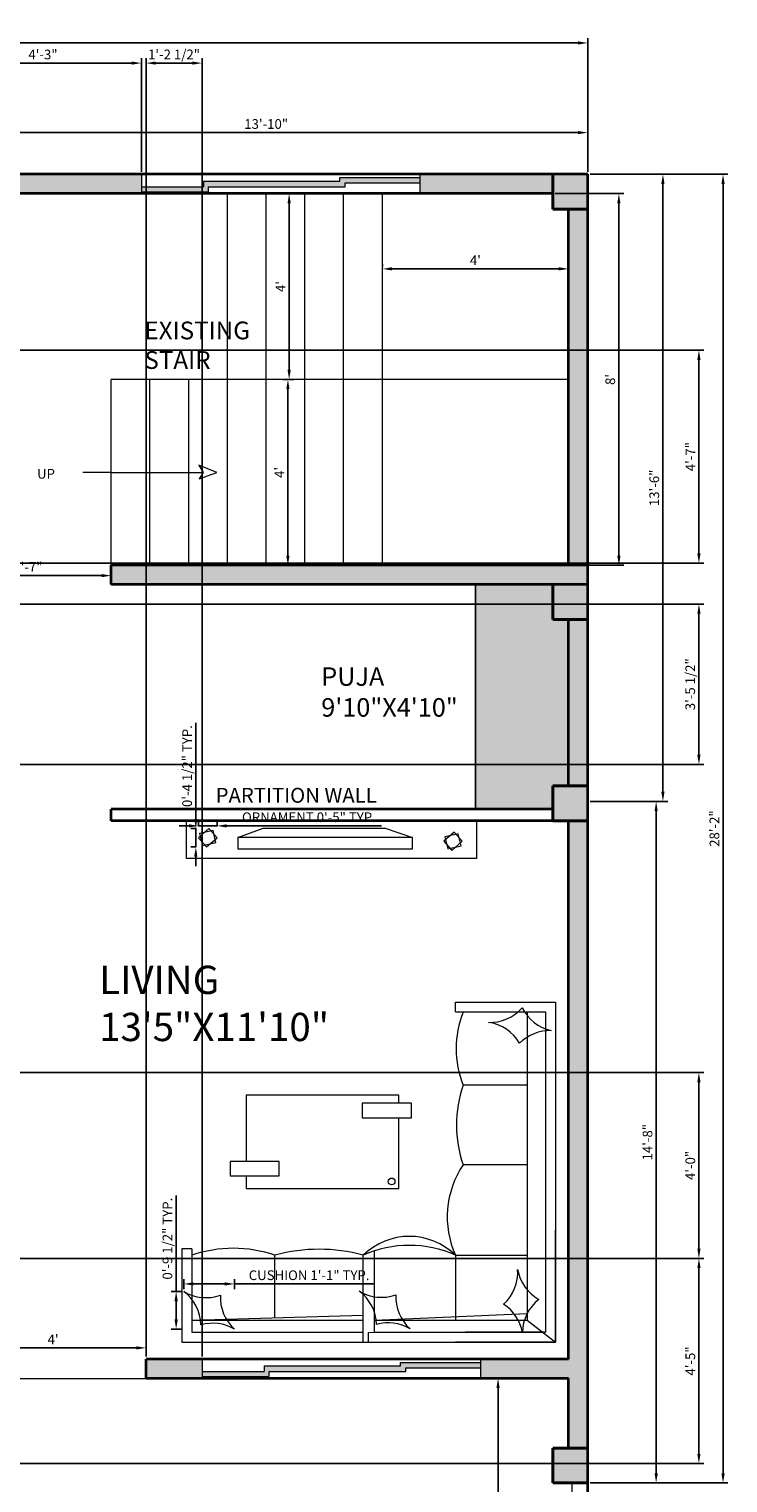
# Model space of a CAD drawing. Units: inches. Extents: x 918 to 1328, y 603 to 1174.
# Tile 4 of 4: x 1147 to 1328, y 798 to 1174. Entities that reach past the tile are written whole.
import ezdxf

# ---------------------------------------------------------------- set-up
doc = ezdxf.new("R2010")
doc.units = ezdxf.units.IN
for name, color, linetype, lineweight in [('A-ANNO-DIMS', 1, 'Continuous', 18), ('A-ANNO-SYMB', 1, 'Continuous', 18), ('A-ANNO-TEXT', 7, 'Continuous', 18), ('A-COLS', 7, 'Continuous', 40), ('A-DOOR', 4, 'Continuous', 18), ('A-FLOR', 7, 'Continuous', 25), ('A-FLOR-CASE', 8, 'Continuous', 20), ('A-FLOR-RAIL', 7, 'Continuous', 18), ('A-FURN', 8, 'Continuous', 18), ('A-GLAZ', 4, 'Continuous', 18), ('A-GLAZ-PATT', 5, 'Continuous', 13), ('A-WALL', 7, 'Continuous', 35), ('A-WALL-PATT', 7, 'Continuous', 13)]:
    doc.layers.add(name, color=color, linetype=linetype, lineweight=lineweight)
for name, color, linetype, lineweight, true_color in [('A-AREA-IDEN', 251, 'Continuous', 20, 0x636466), ('A-COLS-PATT', 251, 'Continuous', 13, 0x636466), ('A-EQPM', 252, 'Continuous', 18, 0x939598), ('A-FLOR-PATT', 40, 'Continuous', 13, 0xf8d731), ('A-FLOR-STRS', 251, 'Continuous', 20, 0x636466)]:
    doc.layers.add(name, color=color, linetype=linetype, lineweight=lineweight, true_color=true_color)
doc.styles.get("Standard").update_dxf_attribs({"font": 'arial.ttf'})
doc.dimstyles.new('ISO-25', dxfattribs={"dimtxt": 2.5, "dimasz": 2.5, "dimexe": 1.25, "dimexo": 0.625, "dimtad": 1, "dimdec": 0, "dimlunit": 3, "dimtxsty": 'Standard', "dimcen": 2.5, "dimadec": 0, "dimazin": 0, "dimtfac": 1, "dimtdec": 0, "dimtmove": 0, "dimatfit": 3, "dimfxl": 1, "dimarcsym": 0})

# ---------------------------------------------------------------- blocks, each defined once
blk = doc.blocks.new('*D1')
at = {"layer": 'A-ANNO-DIMS', "color": 0, "lineweight": -2, "transparency": 16777216}
for p, q in [((956.48, 1136.87), (956.48, 1171.39)), ((958.98, 1170.14), (1288.98, 1170.14)), ((1291.48, 1136.87), (1291.48, 1171.39))]:
    blk.add_line(p, q, dxfattribs=at)
at = {"layer": 'A-ANNO-DIMS', "color": 0, "transparency": 16777216}
for points in [[(958.98, 1170.56), (958.98, 1169.73), (956.48, 1170.14)], [(1288.98, 1170.56), (1288.98, 1169.73), (1291.48, 1170.14)]]:
    blk.add_solid(points, dxfattribs=at)
at = {"layer": 'Defpoints', "color": 0, "transparency": 16777216}
for p in [(1291.48, 1170.14), (956.48, 1136.24), (1291.48, 1136.24)]:
    blk.add_point(p, dxfattribs=at)
at = {"layer": 'A-ANNO-DIMS', "color": 0, "transparency": 16777216, "insert": (1123.98, 1172.02), "char_height": 2.5, "attachment_point": 5}
blk.add_mtext('27\'-11"', dxfattribs=at)
blk = doc.blocks.new('*D4')
at = {"layer": 'A-ANNO-DIMS', "color": 0, "lineweight": -2, "transparency": 16777216}
for p, q in [((1292.11, 1136.24), (1327.66, 1136.24)), ((1326.41, 800.74), (1326.41, 1133.74)), ((1292.11, 798.24), (1327.66, 798.24))]:
    blk.add_line(p, q, dxfattribs=at)
at = {"layer": 'A-ANNO-DIMS', "color": 0, "transparency": 16777216}
for points in [[(1326, 1133.74), (1326.83, 1133.74), (1326.41, 1136.24)], [(1326, 800.74), (1326.83, 800.74), (1326.41, 798.24)]]:
    blk.add_solid(points, dxfattribs=at)
at = {"layer": 'Defpoints', "color": 0, "transparency": 16777216}
for p in [(1291.48, 1136.24), (1326.41, 1136.24), (1291.48, 798.24)]:
    blk.add_point(p, dxfattribs=at)
at = {"layer": 'A-ANNO-DIMS', "color": 0, "transparency": 16777216, "insert": (1324.51, 967.24), "char_height": 2.5, "attachment_point": 5, "rotation": 90}
blk.add_mtext('28\'-2"', dxfattribs=at)
blk = doc.blocks.new('*D5')
at = {"layer": 'A-ANNO-DIMS', "color": 0, "lineweight": -2, "transparency": 16777216}
for p, q in [((1125.48, 1136.87), (1125.48, 1148.24)), ((1127.98, 1146.99), (1288.98, 1146.99)), ((1291.48, 1136.87), (1291.48, 1148.24))]:
    blk.add_line(p, q, dxfattribs=at)
at = {"layer": 'A-ANNO-DIMS', "color": 0, "transparency": 16777216}
for points in [[(1127.98, 1147.4), (1127.98, 1146.57), (1125.48, 1146.99)], [(1288.98, 1147.4), (1288.98, 1146.57), (1291.48, 1146.99)]]:
    blk.add_solid(points, dxfattribs=at)
at = {"layer": 'Defpoints', "color": 0, "transparency": 16777216}
for p in [(1291.48, 1146.99), (1125.48, 1136.24), (1291.48, 1136.24)]:
    blk.add_point(p, dxfattribs=at)
at = {"layer": 'A-ANNO-DIMS', "color": 0, "transparency": 16777216, "insert": (1208.48, 1148.89), "char_height": 2.5, "attachment_point": 5}
blk.add_mtext('13\'-10"', dxfattribs=at)
blk = doc.blocks.new('*D9')
at = {"layer": 'A-ANNO-DIMS', "color": 0, "lineweight": -2, "transparency": 16777216}
for p, q in [((1292.11, 1136.24), (1312.14, 1136.24)), ((1310.89, 976.74), (1310.89, 1133.74)), ((1292.11, 974.24), (1312.14, 974.24))]:
    blk.add_line(p, q, dxfattribs=at)
at = {"layer": 'A-ANNO-DIMS', "color": 0, "transparency": 16777216}
for points in [[(1310.47, 1133.74), (1311.3, 1133.74), (1310.89, 1136.24)], [(1310.47, 976.74), (1311.3, 976.74), (1310.89, 974.24)]]:
    blk.add_solid(points, dxfattribs=at)
at = {"layer": 'Defpoints', "color": 0, "transparency": 16777216}
for p in [(1291.48, 1136.24), (1310.89, 1136.24), (1291.48, 974.24)]:
    blk.add_point(p, dxfattribs=at)
at = {"layer": 'A-ANNO-DIMS', "color": 0, "transparency": 16777216, "insert": (1308.98, 1055.24), "char_height": 2.5, "attachment_point": 5, "rotation": 90}
blk.add_mtext('13\'-6"', dxfattribs=at)
blk = doc.blocks.new('*D10')
at = {"layer": 'A-ANNO-DIMS', "color": 0, "lineweight": -2, "transparency": 16777216}
for p, q in [((1292.11, 974.24), (1310.39, 974.24)), ((1309.14, 971.74), (1309.14, 800.74)), ((1292.11, 798.24), (1310.39, 798.24))]:
    blk.add_line(p, q, dxfattribs=at)
at = {"layer": 'A-ANNO-DIMS', "color": 0, "transparency": 16777216}
for points in [[(1308.73, 971.74), (1309.56, 971.74), (1309.14, 974.24)], [(1308.73, 800.74), (1309.56, 800.74), (1309.14, 798.24)]]:
    blk.add_solid(points, dxfattribs=at)
at = {"layer": 'Defpoints', "color": 0, "transparency": 16777216}
for p in [(1291.48, 974.24), (1291.48, 798.24), (1309.14, 798.24)]:
    blk.add_point(p, dxfattribs=at)
at = {"layer": 'A-ANNO-DIMS', "color": 0, "transparency": 16777216, "insert": (1307.24, 886.24), "char_height": 2.5, "attachment_point": 5, "rotation": 90}
blk.add_mtext('14\'-8"', dxfattribs=at)
blk = doc.blocks.new('*D12')
at = {"layer": 'A-ANNO-DIMS', "color": 0, "lineweight": -2, "transparency": 16777216}
for p, q in [((1283.11, 1131.24), (1300.77, 1131.24)), ((1299.52, 1128.74), (1299.52, 1037.74)), ((1283.11, 1035.24), (1300.77, 1035.24))]:
    blk.add_line(p, q, dxfattribs=at)
at = {"layer": 'A-ANNO-DIMS', "color": 0, "transparency": 16777216}
for points in [[(1299.11, 1128.74), (1299.94, 1128.74), (1299.52, 1131.24)], [(1299.11, 1037.74), (1299.94, 1037.74), (1299.52, 1035.24)]]:
    blk.add_solid(points, dxfattribs=at)
at = {"layer": 'Defpoints', "color": 0, "transparency": 16777216}
for p in [(1282.48, 1131.24), (1282.48, 1035.24), (1299.52, 1035.24)]:
    blk.add_point(p, dxfattribs=at)
at = {"layer": 'A-ANNO-DIMS', "color": 0, "transparency": 16777216, "insert": (1297.62, 1083.24), "char_height": 2.5, "attachment_point": 5, "rotation": 90}
blk.add_mtext("8'", dxfattribs=at)
blk = doc.blocks.new('*D13')
at = {"layer": 'A-ANNO-DIMS', "color": 0, "lineweight": -2, "transparency": 16777216}
for p, q in [((1238.48, 1112.43), (1238.48, 1113.05)), ((1240.98, 1111.8), (1283.98, 1111.8)), ((1286.48, 1112.43), (1286.48, 1113.05))]:
    blk.add_line(p, q, dxfattribs=at)
at = {"layer": 'A-ANNO-DIMS', "color": 0, "transparency": 16777216}
for points in [[(1240.98, 1112.22), (1240.98, 1111.38), (1238.48, 1111.8)], [(1283.98, 1112.22), (1283.98, 1111.38), (1286.48, 1111.8)]]:
    blk.add_solid(points, dxfattribs=at)
at = {"layer": 'Defpoints', "color": 0, "transparency": 16777216}
for p in [(1238.48, 1111.8), (1286.48, 1111.8), (1286.48, 1111.8)]:
    blk.add_point(p, dxfattribs=at)
at = {"layer": 'A-ANNO-DIMS', "color": 0, "transparency": 16777216, "insert": (1262.48, 1113.68), "char_height": 2.5, "attachment_point": 5}
blk.add_mtext("4'", dxfattribs=at)
blk = doc.blocks.new('*D14')
at = {"layer": 'A-ANNO-DIMS', "color": 0, "lineweight": -2, "transparency": 16777216}
for p, q in [((1214.22, 1131.24), (1215.66, 1131.24)), ((1214.41, 1085.74), (1214.41, 1128.74)), ((1214.22, 1083.24), (1215.66, 1083.24))]:
    blk.add_line(p, q, dxfattribs=at)
at = {"layer": 'A-ANNO-DIMS', "color": 0, "transparency": 16777216}
for points in [[(1213.99, 1128.74), (1214.83, 1128.74), (1214.41, 1131.24)], [(1213.99, 1085.74), (1214.83, 1085.74), (1214.41, 1083.24)]]:
    blk.add_solid(points, dxfattribs=at)
at = {"layer": 'Defpoints', "color": 0, "transparency": 16777216}
for p in [(1213.6, 1131.24), (1214.41, 1131.24), (1213.6, 1083.24)]:
    blk.add_point(p, dxfattribs=at)
at = {"layer": 'A-ANNO-DIMS', "color": 0, "transparency": 16777216, "insert": (1212.54, 1107.24), "char_height": 2.5, "attachment_point": 5, "rotation": 90}
blk.add_mtext("4'", dxfattribs=at)
blk = doc.blocks.new('*D15')
at = {"layer": 'A-ANNO-DIMS', "color": 0, "lineweight": -2, "transparency": 16777216}
for p, q in [((1213.79, 1083.24), (1212.84, 1083.24)), ((1214.09, 1080.74), (1214.09, 1037.74)), ((1213.79, 1035.24), (1212.84, 1035.24))]:
    blk.add_line(p, q, dxfattribs=at)
at = {"layer": 'A-ANNO-DIMS', "color": 0, "transparency": 16777216}
for points in [[(1213.67, 1080.74), (1214.5, 1080.74), (1214.09, 1083.24)], [(1213.67, 1037.74), (1214.5, 1037.74), (1214.09, 1035.24)]]:
    blk.add_solid(points, dxfattribs=at)
at = {"layer": 'Defpoints', "color": 0, "transparency": 16777216}
for p in [(1214.41, 1083.24), (1214.09, 1035.24), (1214.41, 1035.24)]:
    blk.add_point(p, dxfattribs=at)
at = {"layer": 'A-ANNO-DIMS', "color": 0, "transparency": 16777216, "insert": (1212.21, 1059.24), "char_height": 2.5, "attachment_point": 5, "rotation": 90}
blk.add_mtext("4'", dxfattribs=at)
blk = doc.blocks.new('*D16')
at = {"layer": 'A-ANNO-DIMS', "color": 0, "lineweight": -2, "transparency": 16777216}
for p, q in [((1125.48, 1033.2), (1125.48, 1033.82)), ((1168.48, 1033.2), (1168.48, 1033.82)), ((1165.98, 1032.57), (1127.98, 1032.57))]:
    blk.add_line(p, q, dxfattribs=at)
at = {"layer": 'A-ANNO-DIMS', "color": 0, "transparency": 16777216}
for points in [[(1127.98, 1032.99), (1127.98, 1032.16), (1125.48, 1032.57)], [(1165.98, 1032.99), (1165.98, 1032.16), (1168.48, 1032.57)]]:
    blk.add_solid(points, dxfattribs=at)
at = {"layer": 'Defpoints', "color": 0, "transparency": 16777216}
for p in [(1125.48, 1032.57), (1125.48, 1032.57), (1168.48, 1032.57)]:
    blk.add_point(p, dxfattribs=at)
at = {"layer": 'A-ANNO-DIMS', "color": 0, "transparency": 16777216, "insert": (1146.98, 1034.48), "char_height": 2.5, "attachment_point": 5}
blk.add_mtext('3\'-7"', dxfattribs=at)
blk = doc.blocks.new('*D17')
at = {"layer": 'A-ANNO-DIMS', "color": 0, "lineweight": -2, "transparency": 16777216}
for p, q in [((1129.48, 830.87), (1129.48, 834.37)), ((1177.48, 830.87), (1177.48, 834.37)), ((1131.98, 833.12), (1174.98, 833.12))]:
    blk.add_line(p, q, dxfattribs=at)
at = {"layer": 'A-ANNO-DIMS', "color": 0, "transparency": 16777216}
for points in [[(1131.98, 833.53), (1131.98, 832.7), (1129.48, 833.12)], [(1174.98, 833.53), (1174.98, 832.7), (1177.48, 833.12)]]:
    blk.add_solid(points, dxfattribs=at)
at = {"layer": 'Defpoints', "color": 0, "transparency": 16777216}
for p in [(1129.48, 830.24), (1177.48, 833.12), (1177.48, 830.24)]:
    blk.add_point(p, dxfattribs=at)
at = {"layer": 'A-ANNO-DIMS', "color": 0, "transparency": 16777216, "insert": (1153.48, 834.99), "char_height": 2.5, "attachment_point": 5}
blk.add_mtext("4'", dxfattribs=at)
blk = doc.blocks.new('*D20')
at = {"layer": 'A-ANNO-DIMS', "color": 0, "lineweight": -2, "transparency": 16777216}
for p, q in [((1272.05, 825.24), (1267.09, 825.24)), ((1268.34, 731.74), (1268.34, 822.74)), ((1272.05, 729.24), (1267.09, 729.24))]:
    blk.add_line(p, q, dxfattribs=at)
at = {"layer": 'A-ANNO-DIMS', "color": 0, "transparency": 16777216}
for points in [[(1267.92, 822.74), (1268.75, 822.74), (1268.34, 825.24)], [(1267.92, 731.74), (1268.75, 731.74), (1268.34, 729.24)]]:
    blk.add_solid(points, dxfattribs=at)
at = {"layer": 'Defpoints', "color": 0, "transparency": 16777216}
for p in [(1268.34, 825.24), (1272.68, 825.24), (1272.68, 729.24)]:
    blk.add_point(p, dxfattribs=at)
at = {"layer": 'A-ANNO-DIMS', "color": 0, "transparency": 16777216, "insert": (1266.44, 777.24), "char_height": 2.5, "attachment_point": 5, "rotation": 90}
blk.add_mtext("8'", dxfattribs=at)
blk = doc.blocks.new('WIN-SLIDING-72')
for p, q in [((0, 5), (0, 0)), ((72, 5), (0, 5)), ((51.22, 4.12), (72, 4.12)), ((51.22, 3.25), (51.22, 4.12)), ((72, 0), (72, 5)), ((0, 1.76), (16, 1.76)), ((0, 0.47), (17.22, 0.47)), ((0, 0), (72, 0)), ((16, 3.25), (51.22, 3.25)), ((16, 3.25), (16, 1.76)), ((17.22, 1.76), (51.22, 1.76)), ((17.22, 1.76), (17.22, 0.47)), ((51.22, 1.76), (52.58, 1.76)), ((52.58, 2.76), (72, 2.76)), ((52.58, 1.76), (52.58, 2.76))]:
    blk.add_line(p, q)
blk = doc.blocks.new('CUSHION-SOFA')
for centre, radius, start, end in [((5.72, 19.23), 11.1, 238.9544, 289.6508), ((-6.51, 0.95), 10.92, 0.7876, 53.4103), ((20.54, 8.23), 11.1, 177.1699, 227.8663), ((7.47, -9.57), 11.1, 59.5445, 105.9983)]:
    blk.add_arc(centre, radius, start, end)
blk = doc.blocks.new('CONSOLE-ORNAMENT')
for p, q in [((2.68, 4.73), (0, 2.4)), ((3.73, 4.29), (0.28, 3.48)), ((4.76, 2.33), (2.68, 4.73)), ((4.46, 1.19), (3.73, 4.29)), ((0, 2.4), (2.08, 0)), ((0.28, 3.48), (1, 0.38)), ((1, 0.38), (4.46, 1.19)), ((2.08, 0), (4.76, 2.33))]:
    blk.add_line(p, q)
blk = doc.blocks.new('*D34')
at = {"layer": 'A-ANNO-DIMS', "color": 0, "lineweight": -2, "transparency": 16777216}
for p, q in [((1187.21, 848.3), (1187.21, 850.89)), ((1189.71, 849.64), (1197.8, 849.64)), ((1200.3, 848.3), (1200.3, 850.89)), ((1200.3, 849.64), (1236.33, 849.64))]:
    blk.add_line(p, q, dxfattribs=at)
at = {"layer": 'A-ANNO-DIMS', "color": 0, "transparency": 16777216}
for points in [[(1189.71, 850.06), (1189.71, 849.22), (1187.21, 849.64)], [(1197.8, 850.06), (1197.8, 849.22), (1200.3, 849.64)]]:
    blk.add_solid(points, dxfattribs=at)
at = {"layer": 'Defpoints', "color": 0, "transparency": 16777216}
for p in [(1200.3, 849.64), (1187.21, 847.68), (1200.3, 847.68)]:
    blk.add_point(p, dxfattribs=at)
at = {"layer": 'A-ANNO-DIMS', "color": 0, "transparency": 16777216, "insert": (1219.57, 851.56), "char_height": 2.5, "attachment_point": 5}
blk.add_mtext('CUSHION 1\'-1" TYP.', dxfattribs=at)
blk = doc.blocks.new('*D35')
at = {"layer": 'A-ANNO-DIMS', "color": 0, "lineweight": -2, "transparency": 16777216}
for p, q in [((1185.24, 847.68), (1185.24, 872.49)), ((1186.58, 847.68), (1183.99, 847.68)), ((1185.24, 840.45), (1185.24, 845.18)), ((1186.58, 837.95), (1183.99, 837.95))]:
    blk.add_line(p, q, dxfattribs=at)
at = {"layer": 'A-ANNO-DIMS', "color": 0, "transparency": 16777216}
for points in [[(1184.82, 845.18), (1185.66, 845.18), (1185.24, 847.68)], [(1184.82, 840.45), (1185.66, 840.45), (1185.24, 837.95)]]:
    blk.add_solid(points, dxfattribs=at)
at = {"layer": 'Defpoints', "color": 0, "transparency": 16777216}
for p in [(1185.24, 847.68), (1187.21, 847.68), (1187.21, 837.95)]:
    blk.add_point(p, dxfattribs=at)
at = {"layer": 'A-ANNO-DIMS', "color": 0, "transparency": 16777216, "insert": (1183.32, 861.33), "char_height": 2.5, "attachment_point": 5, "rotation": 90}
blk.add_mtext('0\'-9 1/2" TYP.', dxfattribs=at)
blk = doc.blocks.new('*D42')
at = {"layer": 'A-ANNO-DIMS', "color": 0, "lineweight": -2, "transparency": 16777216}
for p, q in [((1191.03, 967.85), (1191.03, 969.19)), ((1195.8, 967.85), (1195.8, 969.19)), ((1188.53, 967.94), (1186.03, 967.94)), ((1191.03, 967.94), (1195.8, 967.94)), ((1198.3, 967.94), (1238.22, 967.94))]:
    blk.add_line(p, q, dxfattribs=at)
at = {"layer": 'A-ANNO-DIMS', "color": 0, "transparency": 16777216}
for points in [[(1188.53, 968.35), (1188.53, 967.52), (1191.03, 967.94)], [(1198.3, 968.35), (1198.3, 967.52), (1195.8, 967.94)]]:
    blk.add_solid(points, dxfattribs=at)
at = {"layer": 'Defpoints', "color": 0, "transparency": 16777216}
for p in [(1191.03, 967.22), (1195.8, 967.94), (1195.8, 967.22)]:
    blk.add_point(p, dxfattribs=at)
at = {"layer": 'A-ANNO-DIMS', "color": 0, "transparency": 16777216, "insert": (1219.51, 969.85), "char_height": 2.5, "attachment_point": 5}
blk.add_mtext('ORNAMENT 0\'-5" TYP.', dxfattribs=at)
blk = doc.blocks.new('*D43')
at = {"layer": 'A-ANNO-DIMS', "color": 0, "lineweight": -2, "transparency": 16777216}
for p, q in [((1190.32, 969.72), (1190.32, 994.54)), ((1190.41, 967.22), (1189.07, 967.22)), ((1190.32, 962.49), (1190.32, 967.22)), ((1190.41, 962.49), (1189.07, 962.49)), ((1190.32, 959.99), (1190.32, 957.49))]:
    blk.add_line(p, q, dxfattribs=at)
at = {"layer": 'A-ANNO-DIMS', "color": 0, "transparency": 16777216}
for points in [[(1189.9, 969.72), (1190.73, 969.72), (1190.32, 967.22)], [(1189.9, 959.99), (1190.73, 959.99), (1190.32, 962.49)]]:
    blk.add_solid(points, dxfattribs=at)
at = {"layer": 'Defpoints', "color": 0, "transparency": 16777216}
for p in [(1190.32, 967.22), (1191.03, 967.22), (1191.03, 962.49)]:
    blk.add_point(p, dxfattribs=at)
at = {"layer": 'A-ANNO-DIMS', "color": 0, "transparency": 16777216, "insert": (1188.4, 983.38), "char_height": 2.5, "attachment_point": 5, "rotation": 90}
blk.add_mtext('0\'-4 1/2" TYP.', dxfattribs=at)
blk = doc.blocks.new('*D46')
at = {"layer": 'A-ANNO-DIMS', "color": 0, "lineweight": -2, "transparency": 16777216}
for p, q in [((1125.48, 1136.87), (1125.48, 1166.19)), ((1127.98, 1164.94), (1173.76, 1164.94)), ((1176.26, 1136.87), (1176.26, 1166.19))]:
    blk.add_line(p, q, dxfattribs=at)
at = {"layer": 'A-ANNO-DIMS', "color": 0, "transparency": 16777216}
for points in [[(1127.98, 1165.36), (1127.98, 1164.53), (1125.48, 1164.94)], [(1173.76, 1165.36), (1173.76, 1164.53), (1176.26, 1164.94)]]:
    blk.add_solid(points, dxfattribs=at)
at = {"layer": 'Defpoints', "color": 0, "transparency": 16777216}
for p in [(1176.26, 1164.94), (1125.48, 1136.24), (1176.26, 1136.24)]:
    blk.add_point(p, dxfattribs=at)
at = {"layer": 'A-ANNO-DIMS', "color": 0, "transparency": 16777216, "insert": (1150.87, 1166.84), "char_height": 2.5, "attachment_point": 5}
blk.add_mtext('4\'-3"', dxfattribs=at)
blk = doc.blocks.new('*D49')
at = {"layer": 'A-ANNO-DIMS', "color": 0, "lineweight": -2, "transparency": 16777216}
for p, q in [((1177.48, 830.87), (1177.48, 1166.19)), ((1179.98, 1164.94), (1189.42, 1164.94)), ((1191.92, 830.87), (1191.92, 1166.19))]:
    blk.add_line(p, q, dxfattribs=at)
at = {"layer": 'A-ANNO-DIMS', "color": 0, "transparency": 16777216}
for points in [[(1179.98, 1165.36), (1179.98, 1164.53), (1177.48, 1164.94)], [(1189.42, 1165.36), (1189.42, 1164.53), (1191.92, 1164.94)]]:
    blk.add_solid(points, dxfattribs=at)
at = {"layer": 'Defpoints', "color": 0, "transparency": 16777216}
for p in [(1191.92, 1164.94), (1177.48, 830.24), (1191.92, 830.24)]:
    blk.add_point(p, dxfattribs=at)
at = {"layer": 'A-ANNO-DIMS', "color": 0, "transparency": 16777216, "insert": (1184.7, 1166.86), "char_height": 2.5, "attachment_point": 5}
blk.add_mtext('1\'-2 1/2"', dxfattribs=at)
blk = doc.blocks.new('*D50')
at = {"layer": 'A-ANNO-DIMS', "color": 0, "lineweight": -2, "transparency": 16777216}
for p, q in [((1121.11, 1025.24), (1321.43, 1025.24)), ((1320.18, 1022.74), (1320.18, 986.29)), ((1121.11, 983.79), (1321.43, 983.79))]:
    blk.add_line(p, q, dxfattribs=at)
at = {"layer": 'A-ANNO-DIMS', "color": 0, "transparency": 16777216}
for points in [[(1319.77, 1022.74), (1320.6, 1022.74), (1320.18, 1025.24)], [(1319.77, 986.29), (1320.6, 986.29), (1320.18, 983.79)]]:
    blk.add_solid(points, dxfattribs=at)
at = {"layer": 'Defpoints', "color": 0, "transparency": 16777216}
for p in [(1120.48, 1025.24), (1120.48, 983.79), (1320.18, 983.79)]:
    blk.add_point(p, dxfattribs=at)
at = {"layer": 'A-ANNO-DIMS', "color": 0, "transparency": 16777216, "insert": (1318.26, 1004.52), "char_height": 2.5, "attachment_point": 5, "rotation": 90}
blk.add_mtext('3\'-5 1/2"', dxfattribs=at)
blk = doc.blocks.new('*D51')
at = {"layer": 'A-ANNO-DIMS', "color": 0, "lineweight": -2, "transparency": 16777216}
for p, q in [((1126.11, 904.24), (1321.43, 904.24)), ((1320.18, 901.74), (1320.18, 858.74)), ((1126.11, 856.24), (1321.43, 856.24))]:
    blk.add_line(p, q, dxfattribs=at)
at = {"layer": 'A-ANNO-DIMS', "color": 0, "transparency": 16777216}
for points in [[(1319.77, 901.74), (1320.6, 901.74), (1320.18, 904.24)], [(1319.77, 858.74), (1320.6, 858.74), (1320.18, 856.24)]]:
    blk.add_solid(points, dxfattribs=at)
at = {"layer": 'Defpoints', "color": 0, "transparency": 16777216}
for p in [(1125.48, 904.24), (1125.48, 856.24), (1320.18, 856.24)]:
    blk.add_point(p, dxfattribs=at)
at = {"layer": 'A-ANNO-DIMS', "color": 0, "transparency": 16777216, "insert": (1318.28, 880.24), "char_height": 2.5, "attachment_point": 5, "rotation": 90}
blk.add_mtext('4\'-0"', dxfattribs=at)
blk = doc.blocks.new('*D53')
at = {"layer": 'A-ANNO-DIMS', "color": 0, "lineweight": -2, "transparency": 16777216}
for p, q in [((1036.99, 1090.79), (1321.43, 1090.79)), ((1320.18, 1038.3), (1320.18, 1088.29)), ((1036.99, 1035.8), (1321.43, 1035.8))]:
    blk.add_line(p, q, dxfattribs=at)
at = {"layer": 'A-ANNO-DIMS', "color": 0, "transparency": 16777216}
for points in [[(1319.77, 1088.29), (1320.6, 1088.29), (1320.18, 1090.79)], [(1319.77, 1038.3), (1320.6, 1038.3), (1320.18, 1035.8)]]:
    blk.add_solid(points, dxfattribs=at)
at = {"layer": 'Defpoints', "color": 0, "transparency": 16777216}
for p in [(1036.36, 1090.79), (1320.18, 1090.79), (1036.36, 1035.8)]:
    blk.add_point(p, dxfattribs=at)
at = {"layer": 'A-ANNO-DIMS', "color": 0, "transparency": 16777216, "insert": (1318.31, 1063.3), "char_height": 2.5, "attachment_point": 5, "rotation": 90}
blk.add_mtext('4\'-7"', dxfattribs=at)
blk = doc.blocks.new('*D56')
at = {"layer": 'A-ANNO-DIMS', "color": 0, "lineweight": -2, "transparency": 16777216}
for p, q in [((1082.11, 856.24), (1321.43, 856.24)), ((1320.18, 853.74), (1320.18, 805.74)), ((1082.11, 803.24), (1321.43, 803.24))]:
    blk.add_line(p, q, dxfattribs=at)
at = {"layer": 'A-ANNO-DIMS', "color": 0, "transparency": 16777216}
for points in [[(1319.77, 853.74), (1320.6, 853.74), (1320.18, 856.24)], [(1319.77, 805.74), (1320.6, 805.74), (1320.18, 803.24)]]:
    blk.add_solid(points, dxfattribs=at)
at = {"layer": 'Defpoints', "color": 0, "transparency": 16777216}
for p in [(1081.48, 856.24), (1081.48, 803.24), (1320.18, 803.24)]:
    blk.add_point(p, dxfattribs=at)
at = {"layer": 'A-ANNO-DIMS', "color": 0, "transparency": 16777216, "insert": (1318.29, 829.74), "char_height": 2.5, "attachment_point": 5, "rotation": 90}
blk.add_mtext('4\'-5"', dxfattribs=at)

msp = doc.modelspace()

# ---------------------------------------------------------------- hatches: boundary and pattern name
at = {"layer": 'A-COLS-PATT'}
h = msp.add_hatch(color=256, dxfattribs=at)
h.dxf.hatch_style = 1
h.paths.add_polyline_path([(965.48, 1136.24), (956.48, 1136.24), (956.48, 1127.24), (965.48, 1127.24)])
h.paths.add_polyline_path([(1125.48, 1136.24), (1116.48, 1136.24), (1116.48, 1127.24), (1125.48, 1127.24)])
h.paths.add_polyline_path([(1291.48, 1136.24), (1282.48, 1136.24), (1282.48, 1127.24), (1291.48, 1127.24)])
h.paths.add_polyline_path([(1125.48, 978.24), (1116.48, 978.24), (1116.48, 969.24), (1125.48, 969.24)])
h.paths.add_polyline_path([(965.48, 978.24), (956.48, 978.24), (956.48, 969.24), (965.48, 969.24)])
h.paths.add_polyline_path([(965.48, 807.24), (956.48, 807.24), (956.48, 798.24), (965.48, 798.24)])
h.paths.add_polyline_path([(1125.48, 807.24), (1116.48, 807.24), (1116.48, 798.24), (1125.48, 798.24)])
h.paths.add_polyline_path([(1291.48, 807.24), (1282.48, 807.24), (1282.48, 798.24), (1291.48, 798.24)])
h.paths.add_polyline_path([(1291.48, 1030.24), (1282.48, 1030.24), (1282.48, 1021.24), (1291.48, 1021.24)])
h.paths.add_polyline_path([(1291.48, 978.24), (1282.48, 978.24), (1282.48, 969.24), (1291.48, 969.24)])
at = {"layer": 'A-FLOR-PATT'}
h = msp.add_hatch(color=256, dxfattribs=at)
h.dxf.hatch_style = 1
h.paths.add_polyline_path([(1286.48, 1021.24), (1282.48, 1021.24), (1282.48, 1030.24), (1262.48, 1030.24), (1262.48, 972.24), (1282.48, 972.24), (1282.48, 978.24), (1286.48, 978.24)])
at = {"layer": 'A-GLAZ-PATT'}
h = msp.add_hatch(color=256, dxfattribs=at)
h.dxf.hatch_style = 1
h.paths.add_polyline_path([(1057.57, 1134.01), (1076.98, 1134.01), (1076.98, 1135.36), (1056.2, 1135.36), (1056.2, 1134.49), (1020.98, 1134.49), (1020.98, 1133), (1004.98, 1133), (1004.98, 1131.71), (1022.21, 1131.71), (1022.21, 1133), (1056.21, 1133), (1057.57, 1133)])
h.paths.add_polyline_path([(1228.84, 1134.01), (1248.26, 1134.01), (1248.26, 1135.36), (1227.48, 1135.36), (1227.48, 1134.49), (1192.26, 1134.49), (1192.26, 1133), (1176.26, 1133), (1176.26, 1131.71), (1193.48, 1131.71), (1193.48, 1133), (1227.48, 1133), (1228.84, 1133)])
h.paths.add_polyline_path([(1244.5, 828.01), (1263.92, 828.01), (1263.92, 829.36), (1243.14, 829.36), (1243.14, 828.49), (1207.92, 828.49), (1207.92, 827), (1191.92, 827), (1191.92, 825.71), (1209.14, 825.71), (1209.14, 827), (1243.14, 827), (1244.5, 827)])
at = {"layer": 'A-WALL-PATT'}
h = msp.add_hatch(color=256, dxfattribs=at)
h.dxf.hatch_style = 1
h.paths.add_polyline_path([(961.48, 969.24), (956.48, 969.24), (956.48, 807.24), (961.48, 807.24), (961.48, 904.24), (1125.48, 904.24), (1125.48, 909.24), (1086.48, 909.24), (1086.48, 913.24), (1081.48, 913.24), (1081.48, 909.24), (961.48, 909.24)])
h.paths.add_polyline_path([(1116.48, 974.24), (965.48, 974.24), (965.48, 969.24), (1081.48, 969.24), (1081.48, 943.24), (1086.48, 943.24), (1086.48, 969.24), (1116.48, 969.24)])
h.paths.add_polyline_path([(1004.98, 1136.24), (965.48, 1136.24), (965.48, 1131.24), (1004.98, 1131.24)])
h.paths.add_polyline_path([(1116.48, 1136.24), (1076.98, 1136.24), (1076.98, 1131.24), (1116.48, 1131.24)])
h.paths.add_polyline_path([(1176.26, 1136.24), (1125.48, 1136.24), (1125.48, 1131.24), (1176.26, 1131.24)])
h.paths.add_polyline_path([(1282.48, 1136.24), (1248.26, 1136.24), (1248.26, 1131.24), (1282.48, 1131.24)])
h.paths.add_polyline_path([(1125.48, 1127.24), (1120.48, 1127.24), (1120.48, 1025.24), (1125.48, 1025.24)])
h.paths.add_polyline_path([(1291.48, 1035.24), (1168.48, 1035.24), (1168.48, 1030.24), (1291.48, 1030.24)])
h.paths.add_polyline_path([(1125.48, 825.24), (1129.48, 825.24), (1129.48, 830.24), (1125.48, 830.24), (1125.48, 856.24), (1120.48, 856.24), (1120.48, 807.24), (1125.48, 807.24)])
h.paths.add_polyline_path([(1191.92, 830.24), (1177.48, 830.24), (1177.48, 825.24), (1191.92, 825.24)])
h.paths.add_polyline_path([(1291.48, 969.24), (1286.48, 969.24), (1286.48, 830.24), (1263.92, 830.24), (1263.92, 825.24), (1286.48, 825.24), (1286.48, 807.24), (1291.48, 807.24)])
h.paths.add_polyline_path([(1291.48, 1021.24), (1286.48, 1021.24), (1286.48, 978.24), (1291.48, 978.24)])
h.paths.add_polyline_path([(1291.48, 1127.24), (1286.48, 1127.24), (1286.48, 1035.24), (1291.48, 1035.24)])

# ---------------------------------------------------------------- linework, layer by layer
at = {"layer": 'A-ANNO-SYMB'}
for p, q in [((1168.48, 1059.24), (1161.17, 1059.24)), ((1168.48, 1059.24), (1192.21, 1059.24)), ((1195.76, 1059.24), (1191.08, 1061.13)), ((1191.08, 1061.13), (1192.21, 1059.24)), ((1192.21, 1059.24), (1191.18, 1057.53)), ((1191.18, 1057.53), (1195.76, 1059.24))]:
    msp.add_line(p, q, dxfattribs=at)
at = {"layer": 'A-COLS'}
for p, q in [((1282.48, 1136.24), (1282.48, 1127.24)), ((1282.48, 1127.24), (1291.48, 1127.24)), ((1282.48, 1030.24), (1282.48, 1021.24)), ((1282.48, 1021.24), (1291.48, 1021.24)), ((1291.48, 978.24), (1282.48, 978.24)), ((1282.48, 978.24), (1282.48, 969.24)), ((1282.48, 969.24), (1291.48, 969.24)), ((1291.48, 807.24), (1282.48, 807.24)), ((1282.48, 807.24), (1282.48, 798.24)), ((1282.48, 798.24), (1291.48, 798.24))]:
    msp.add_line(p, q, dxfattribs=at)
at = {"layer": 'A-DOOR'}
msp.add_line((1129.48, 825.24), (1177.48, 825.24), dxfattribs=at)
at = {"layer": 'A-EQPM'}
for p, q in [((1201.14, 964.92), (1207.71, 967.35)), ((1207.71, 967.35), (1239.18, 967.35)), ((1239.18, 967.35), (1246.22, 964.92)), ((1246.22, 964.92), (1201.14, 964.92)), ((1201.14, 964.92), (1201.14, 961.97)), ((1201.14, 961.97), (1246.22, 961.97)), ((1246.22, 961.97), (1246.22, 964.92))]:
    msp.add_line(p, q, dxfattribs=at)
at = {"layer": 'A-FLOR'}
msp.add_line((1262.48, 972.24), (1262.48, 1030.24), dxfattribs=at)
at = {"layer": 'A-FLOR-CASE'}
for p, q in [((1187.88, 969.24), (1262.81, 969.24)), ((1187.88, 959.53), (1187.88, 969.24)), ((1262.81, 969.24), (1262.81, 959.53)), ((1262.81, 959.53), (1187.88, 959.53))]:
    msp.add_line(p, q, dxfattribs=at)
at = {"layer": 'A-FLOR-RAIL'}
msp.add_line((1287.48, 729.24), (1287.48, 798.24), dxfattribs=at)
at = {"layer": 'A-FLOR-STRS'}
for p, q in [((1198.48, 1035.24), (1198.48, 1131.24)), ((1208.48, 1035.24), (1208.48, 1131.24)), ((1218.48, 1035.24), (1218.48, 1131.24)), ((1228.48, 1035.24), (1228.48, 1131.24)), ((1238.48, 1035.24), (1238.48, 1131.24)), ((1168.48, 1035.24), (1168.48, 1083.24)), ((1286.48, 1083.24), (1168.48, 1083.24)), ((1178.48, 1035.24), (1178.48, 1083.24)), ((1188.48, 1035.24), (1188.48, 1083.24))]:
    msp.add_line(p, q, dxfattribs=at)
at = {"layer": 'A-FURN'}
for p, q in [((1257.37, 919.87), (1280.59, 919.87)), ((1275.84, 919.87), (1275.84, 840.27)), ((1280.59, 919.87), (1280.59, 837.18)), ((1275.84, 900.96), (1259.34, 900.96)), ((1275.84, 880.39), (1259.34, 880.39)), ((1283.14, 834.63), (1283.14, 863.56)), ((1186.72, 858.66), (1186.72, 834.63)), ((1189.28, 858.66), (1186.72, 858.66)), ((1189.28, 858.66), (1189.28, 837.18)), ((1210.75, 840.88), (1210.75, 857.04)), ((1233.53, 834.63), (1233.53, 857.04)), ((1236.41, 837.18), (1236.41, 858.15)), ((1257.37, 857.04), (1257.37, 840.27)), ((1257.37, 857.04), (1275.84, 857.04)), ((1189.28, 840.27), (1233.53, 841.53)), ((1236.41, 840.27), (1275.84, 841.98)), ((1189.28, 840.27), (1233.53, 840.27)), ((1236.41, 840.27), (1275.84, 840.27)), ((1275.84, 840.27), (1283.14, 834.63)), ((1186.72, 834.63), (1283.14, 834.63)), ((1189.28, 837.18), (1233.53, 837.18)), ((1234.93, 837.08), (1236.41, 837.18)), ((1234.93, 834.63), (1234.93, 837.08)), ((1236.41, 837.18), (1280.59, 837.18)), ((1280.59, 837.18), (1259.92, 837.18))]:
    msp.add_line(p, q, dxfattribs=at)
for points in [[(1257.37, 919.87), (1257.37, 922.42), (1283.14, 922.42), (1283.14, 834.63), (1257.37, 834.63)], [(1242.69, 896.29), (1242.69, 898.37), (1203.31, 898.37), (1203.31, 881.29)], [(1203.31, 877.52), (1203.31, 874.26), (1242.69, 874.26), (1242.69, 892.52)]]:
    msp.add_lwpolyline(points, dxfattribs=at)
for points in [[(1233.3, 892.52), (1245.96, 892.52), (1245.96, 896.29), (1233.3, 896.29)], [(1199.17, 877.52), (1211.82, 877.52), (1211.82, 881.29), (1199.17, 881.29)]]:
    msp.add_lwpolyline(points, close=True, dxfattribs=at)
msp.add_circle((1240.87, 876.12), 0.859, dxfattribs=at)
for centre, radius, start, end in [((1282.88, 910.41), 25.37, 158.1129, 201.8871), ((1289.12, 890.67), 31.5, 160.9494, 199.0506), ((1279.08, 866.97), 23.87, 145.7823, 204.5802), ((1245.45, 844.96), 16.96, 45.366, 134.634), ((1200.01, 826.22), 32.63, 70.7887, 109.2113), ((1222.14, 815.88), 42.71, 74.5305, 105.4695), ((1245.45, 830.59), 29.01, 65.7447, 114.2553)]:
    msp.add_arc(centre, radius, start, end, dxfattribs=at)
at = {"layer": 'A-WALL'}
for p, q in [((1291.48, 1136.24), (956.48, 1136.24)), ((1291.48, 729.24), (1291.48, 1136.24)), ((1282.48, 1131.24), (1125.48, 1131.24)), ((1286.48, 1035.24), (1286.48, 1127.24)), ((1291.48, 1035.24), (1168.48, 1035.24)), ((1168.48, 1030.24), (1168.48, 1035.24)), ((1291.48, 1030.24), (1168.48, 1030.24)), ((1286.48, 978.24), (1286.48, 1021.24)), ((1282.48, 972.24), (1168.48, 972.24)), ((1168.48, 969.24), (1168.48, 972.24)), ((1282.48, 969.24), (1168.48, 969.24)), ((1291.48, 969.24), (1286.48, 969.24)), ((1286.48, 830.24), (1286.48, 969.24)), ((1286.48, 830.24), (1177.48, 830.24)), ((1177.48, 825.24), (1177.48, 830.24)), ((1286.48, 825.24), (1177.48, 825.24)), ((1286.48, 807.24), (1286.48, 825.24))]:
    msp.add_line(p, q, dxfattribs=at)

# ---------------------------------------------------------------- block references
at = {"layer": 'A-FURN'}
for name, p in [('CONSOLE-ORNAMENT', (1191.03, 962.49)), ('CONSOLE-ORNAMENT', (1254.34, 961.62)), ('CUSHION-SOFA', (1187.2, 837.96)), ('CUSHION-SOFA', (1232.52, 838.05))]:
    msp.add_blockref(name, p, dxfattribs=at)
for p, rotation in [((1270.59, 908.69), 29.13263599710439), ((1266.04, 847.03), 310.8513241123862)]:
    msp.add_blockref('CUSHION-SOFA', p, dxfattribs=dict(at, rotation=rotation))
at = {"layer": 'A-GLAZ'}
for p in [(1176.26, 1131.24), (1191.92, 825.24)]:
    msp.add_blockref('WIN-SLIDING-72', p, dxfattribs=at)

# ---------------------------------------------------------------- texts
at = {"layer": 'A-ANNO-TEXT', "attachment_point": 1}
for s, width, gutter_width, insert, char_height in [('UP', 9.5858, 12.5, (1149.34, 1060.12), 2.5), ('PARTITION WALL', 100.0273, 19.24, (1195.44, 977.76), 3.849)]:
    msp.add_mtext_dynamic_manual_height_columns(s, width=width, gutter_width=gutter_width, heights=[0], dxfattribs=dict(at, insert=insert, char_height=char_height))
at = {"layer": 'A-AREA-IDEN', "attachment_point": 1}
for s, width, gutter_width, insert, char_height in [('EXISTING STAIR', 36.0801, 22.93, (1177.05, 1098.19), 4.5859), ('PUJA\\P9\'10"X4\'10"', 47.8552, 23.89, (1222.7, 1008.89), 4.7778), ('LIVING\\P13\'5"X11\'10"', 213.7118, 36.49, (1165.36, 931.82), 7.2976)]:
    msp.add_mtext_dynamic_manual_height_columns(s, width=width, gutter_width=gutter_width, heights=[0], dxfattribs=dict(at, insert=insert, char_height=char_height))

# ---------------------------------------------------------------- dimensions: what is measured, and where the dimension line sits
at = {"layer": 'A-ANNO-DIMS'}
for base, p1, p2, override, picture, middle in [((1291.48, 1170.14), (956.48, 1136.24), (1291.48, 1136.24), {"dimclrd": 0, "dimclre": 0, "dimclrt": 0}, '*D1', (1123.98, 1172.02)), ((1176.26, 1164.94), (1125.48, 1136.24), (1176.26, 1136.24), {"dimdec": 1, "dimlfac": 1, "dimrnd": 0, "dimzin": 1, "dimdsep": 46, "dimlunit": 4, "dimfrac": 2}, '*D46', (1150.87, 1166.84)), ((1191.92, 1164.94), (1177.48, 830.24), (1191.92, 830.24), {"dimdec": 1, "dimlfac": 1, "dimrnd": 0, "dimzin": 1, "dimdsep": 46, "dimlunit": 4, "dimfrac": 2}, '*D49', (1184.7, 1166.86)), ((1291.48, 1146.99), (1125.48, 1136.24), (1291.48, 1136.24), {"dimclrd": 0, "dimclre": 0, "dimclrt": 0}, '*D5', (1208.48, 1148.89)), ((1286.48, 1111.8), (1238.48, 1111.8), (1286.48, 1111.8), {"dimclrd": 0, "dimclre": 0, "dimclrt": 0}, '*D13', (1262.48, 1113.68)), ((1125.48, 1032.57), (1168.48, 1032.57), (1125.48, 1032.57), {"dimclrd": 0, "dimclre": 0, "dimclrt": 0}, '*D16', (1146.98, 1034.48)), ((1177.48, 833.12), (1129.48, 830.24), (1177.48, 830.24), {"dimclrd": 0, "dimclre": 0, "dimclrt": 0}, '*D17', (1153.48, 834.99))]:
    dim = msp.add_linear_dim(base=base, p1=p1, p2=p2, dimstyle='ISO-25', override=override, dxfattribs=at)
    dim.commit()
    dim.dimension.update_dxf_attribs({"geometry": picture, "text_midpoint": middle})
for base, p1, p2, override, picture, middle in [((1326.41, 1136.24), (1291.48, 798.24), (1291.48, 1136.24), {"dimclrd": 0, "dimclre": 0, "dimclrt": 0}, '*D4', (1324.51, 967.24)), ((1310.89, 1136.24), (1291.48, 974.24), (1291.48, 1136.24), {"dimclrd": 0, "dimclre": 0, "dimclrt": 0}, '*D9', (1308.98, 1055.24)), ((1214.41, 1131.24), (1213.6, 1083.24), (1213.6, 1131.24), {"dimclrd": 0, "dimclre": 0, "dimclrt": 0}, '*D14', (1212.54, 1107.24)), ((1299.52, 1035.24), (1282.48, 1131.24), (1282.48, 1035.24), {"dimclrd": 0, "dimclre": 0, "dimclrt": 0}, '*D12', (1297.62, 1083.24)), ((1320.18, 1090.79), (1036.36, 1035.8), (1036.36, 1090.79), {"dimdec": 1, "dimlfac": 1, "dimrnd": 0, "dimzin": 1, "dimdsep": 46, "dimlunit": 4, "dimfrac": 2}, '*D53', (1318.31, 1063.3)), ((1214.09, 1035.24), (1214.41, 1083.24), (1214.41, 1035.24), {"dimclrd": 0, "dimclre": 0, "dimclrt": 0}, '*D15', (1212.21, 1059.24)), ((1320.1824, 983.7934), (1120.4824, 1025.2425), (1120.4824, 983.7934), {"dimdec": 1, "dimlfac": 1, "dimrnd": 0, "dimzin": 1, "dimdsep": 46, "dimlunit": 4, "dimfrac": 2}, '*D50', (1318.2639, 1004.518)), ((1309.14, 798.24), (1291.48, 974.24), (1291.48, 798.24), {"dimclrd": 0, "dimclre": 0, "dimclrt": 0}, '*D10', (1307.24, 886.24)), ((1320.18, 856.24), (1125.48, 904.24), (1125.48, 856.24), {"dimdec": 1, "dimlfac": 1, "dimrnd": 0, "dimzin": 1, "dimdsep": 46, "dimlunit": 4, "dimfrac": 2}, '*D51', (1318.28, 880.24)), ((1320.18, 803.24), (1081.48, 856.24), (1081.48, 803.24), {"dimdec": 1, "dimlfac": 1, "dimrnd": 0, "dimzin": 1, "dimdsep": 46, "dimlunit": 4, "dimfrac": 2}, '*D56', (1318.29, 829.74)), ((1268.34, 825.24), (1272.68, 729.24), (1272.68, 825.24), {"dimclrd": 0, "dimclre": 0, "dimclrt": 0}, '*D20', (1266.44, 777.24))]:
    dim = msp.add_linear_dim(base=base, p1=p1, p2=p2, angle=90, dimstyle='ISO-25', override=override, dxfattribs=at)
    dim.commit()
    dim.dimension.update_dxf_attribs({"geometry": picture, "text_midpoint": middle})
for base, p1, p2, picture, middle in [((1190.32, 967.22), (1191.03, 962.49), (1191.03, 967.22), '*D43', (1188.4, 983.38)), ((1185.24, 847.68), (1187.21, 837.95), (1187.21, 847.68), '*D35', (1183.32, 861.33))]:
    dim = msp.add_linear_dim(base=base, p1=p1, p2=p2, angle=90, text='<> TYP.', dimstyle='ISO-25', override={"dimdec": 1, "dimlfac": 1, "dimrnd": 0, "dimzin": 1, "dimdsep": 46, "dimlunit": 4, "dimfrac": 2}, dxfattribs=at)
    dim.commit()
    dim.dimension.update_dxf_attribs({"geometry": picture, "text_midpoint": middle})
for base, p1, p2, text, picture, middle in [((1195.8, 967.94), (1191.03, 967.22), (1195.8, 967.22), 'ORNAMENT <> TYP.', '*D42', (1219.51, 969.85)), ((1200.3, 849.64), (1187.21, 847.68), (1200.3, 847.68), 'CUSHION <> TYP.', '*D34', (1219.57, 851.56))]:
    dim = msp.add_linear_dim(base=base, p1=p1, p2=p2, text=text, dimstyle='ISO-25', override={"dimdec": 1, "dimlfac": 1, "dimrnd": 0, "dimzin": 1, "dimdsep": 46, "dimlunit": 4, "dimfrac": 2}, dxfattribs=at)
    dim.commit()
    dim.dimension.update_dxf_attribs({"geometry": picture, "text_midpoint": middle})

doc.saveas('drawing.dxf')
